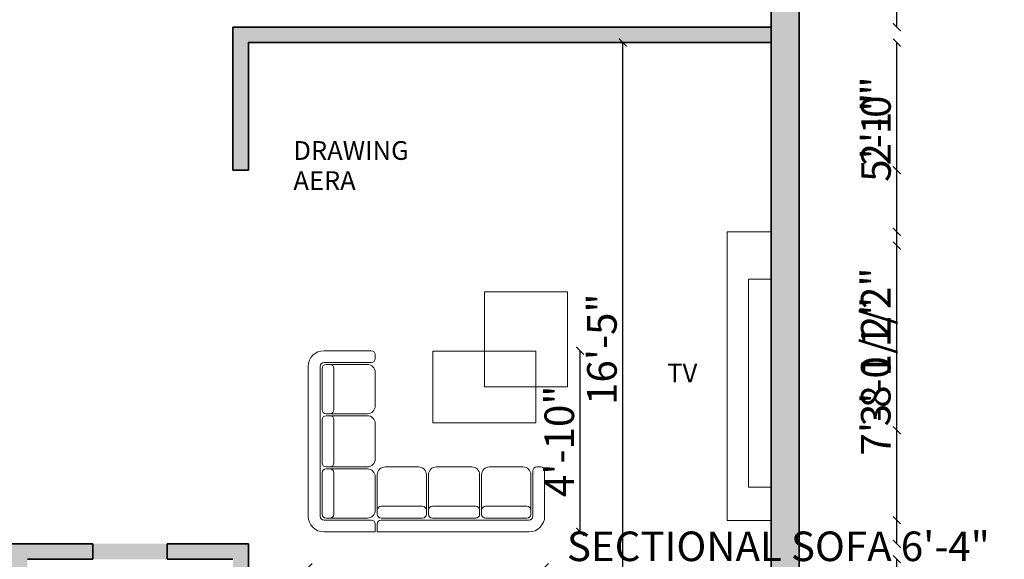
# Model space of a CAD drawing. Units: inches. Extents: x 1704 to 2334, y 1856 to 2559.
# Tile 7 of 10: x 1925 to 2241, y 2148 to 2321. Entities that reach past the tile are written whole.
import ezdxf

# ---------------------------------------------------------------- set-up
doc = ezdxf.new("R2010")
doc.units = ezdxf.units.IN
for name, color, linetype, lineweight in [('A-ANNO-DIMS', 2, 'Continuous', 18), ('A-ANNO-TEXT', 7, 'Continuous', 18), ('A-AREA-IDEN', 7, 'Continuous', 18), ('A-FURN', 8, 'Continuous', 18), ('A-WALL', 7, 'Continuous', 35)]:
    doc.layers.add(name, color=color, linetype=linetype, lineweight=lineweight)
doc.layers.add('A-WALL-PATT', color=18, linetype='Continuous', lineweight=13, true_color=0x000000)
doc.styles.get("Standard").update_dxf_attribs({"font": 'arial.ttf'})
doc.dimstyles.new('ISO-25', dxfattribs={"dimtxt": 9.5, "dimasz": 2.5, "dimexe": 1.25, "dimexo": 0.625, "dimtad": 1, "dimdec": 0, "dimlunit": 4, "dimtxsty": 'Standard', "dimblk": 'ARCHTICK', "dimcen": 2.5, "dimse1": 1, "dimse2": 1, "dimclrd": 3, "dimadec": 0, "dimazin": 0, "dimtfac": 1, "dimtdec": 0, "dimtmove": 0, "dimatfit": 3, "dimfxl": 1, "dimarcsym": 0})

# ---------------------------------------------------------------- blocks, each defined once
blk = doc.blocks.new('A$C2AFA021D')
for p, q in [((0.8, 2.3), (0.2, 2.3)), ((0.85, 2.2), (0.85, 2.25)), ((0.2, 2.15), (0.8, 2.15)), ((0.225, 2.125), (0.275, 2.125)), ((0.75, 2.125), (0.275, 2.125)), ((0, 2.1), (0, 0.2)), ((0.15, 0.2), (0.15, 2.1)), ((0.175, 1.55), (0.175, 2.075)), ((0.325, 2.075), (0.325, 1.55)), ((0.85, 1.6), (0.85, 2.025)), ((0.275, 1.5), (0.225, 1.5)), ((0.275, 1.5), (0.75, 1.5)), ((0.175, 0.875), (0.175, 1.425)), ((0.225, 1.475), (0.275, 1.475)), ((0.75, 1.475), (0.275, 1.475)), ((0.325, 1.425), (0.325, 0.875)), ((0.85, 0.925), (0.85, 1.375)), ((0.175, 0.225), (0.175, 0.75)), ((0.275, 0.825), (0.225, 0.825)), ((0.225, 0.8), (0.275, 0.8)), ((0.275, 0.825), (0.75, 0.825)), ((0.75, 0.8), (0.275, 0.8)), ((0.325, 0.75), (0.325, 0.225)), ((0.975, 0.825), (1.4, 0.825)), ((1.625, 0.825), (2.075, 0.825)), ((2.3, 0.825), (2.725, 0.825)), ((2.85, 0.2), (2.85, 0.775)), ((2.9, 0.825), (2.95, 0.825)), ((3, 0.775), (3, 0.2)), ((0.85, 0.275), (0.85, 0.7)), ((0.875, 0.275), (0.875, 0.725)), ((1.5, 0.725), (1.5, 0.275)), ((1.525, 0.275), (1.525, 0.725)), ((2.175, 0.725), (2.175, 0.275)), ((2.2, 0.275), (2.2, 0.725)), ((2.825, 0.725), (2.825, 0.275)), ((0.875, 0.275), (0.875, 0.225)), ((1.45, 0.325), (0.925, 0.325)), ((1.5, 0.225), (1.5, 0.275)), ((1.525, 0.275), (1.525, 0.225)), ((2.125, 0.325), (1.575, 0.325)), ((2.175, 0.225), (2.175, 0.275)), ((2.2, 0.275), (2.2, 0.225)), ((2.775, 0.325), (2.25, 0.325)), ((2.825, 0.225), (2.825, 0.275)), ((0.8, 0.15), (0.2, 0.15)), ((0.275, 0.175), (0.225, 0.175)), ((0.275, 0.175), (0.75, 0.175)), ((0.925, 0.175), (1.45, 0.175)), ((0.925, 0.15), (2.8, 0.15)), ((1.575, 0.175), (2.125, 0.175)), ((2.25, 0.175), (2.775, 0.175)), ((0.85, 0), (0.85, 0.1)), ((0.875, 0.1), (0.875, 0)), ((0.2, 0), (0.85, 0)), ((2.8, 0), (0.875, 0))]:
    blk.add_line(p, q)
for centre, radius, start, end in [((0.2, 2.1), 0.2, 90, 180), ((0.8, 2.25), 0.05, 0, 90), ((0.2, 2.1), 0.05, 90, 180), ((0.225, 2.075), 0.05, 90, 180), ((0.275, 2.075), 0.05, 0, 90), ((0.75, 2.025), 0.1, 0, 90), ((0.8, 2.2), 0.05, 270, 0), ((0.225, 1.55), 0.05, 180, 270), ((0.275, 1.55), 0.05, 270, 0), ((0.75, 1.6), 0.1, 270, 0), ((0.225, 1.425), 0.05, 90, 180), ((0.275, 1.425), 0.05, 0, 90), ((0.75, 1.375), 0.1, 360, 90), ((0.225, 0.875), 0.05, 180, 270), ((0.275, 0.875), 0.05, 270, 0), ((0.75, 0.925), 0.1, 270, 0), ((0.225, 0.75), 0.05, 90, 180), ((0.275, 0.75), 0.05, 0, 90), ((0.75, 0.7), 0.1, 0, 90), ((0.975, 0.725), 0.1, 90, 180), ((1.4, 0.725), 0.1, 0, 90), ((1.625, 0.725), 0.1, 90, 180), ((2.075, 0.725), 0.1, 0, 90), ((2.3, 0.725), 0.1, 90, 180), ((2.725, 0.725), 0.1, 0, 90), ((2.9, 0.775), 0.05, 90, 180), ((2.95, 0.775), 0.05, 0, 90), ((0.75, 0.275), 0.1, 270, 0), ((0.925, 0.275), 0.05, 90, 180), ((1.45, 0.275), 0.05, 360, 90), ((1.575, 0.275), 0.05, 90, 180), ((2.125, 0.275), 0.05, 360, 90), ((2.25, 0.275), 0.05, 90, 180), ((2.775, 0.275), 0.05, 360, 90), ((0.2, 0.2), 0.2, 180, 270), ((0.2, 0.2), 0.05, 180, 270), ((0.225, 0.225), 0.05, 180, 270), ((0.275, 0.225), 0.05, 270, 0), ((0.8, 0.1), 0.05, 0, 90), ((0.925, 0.225), 0.05, 180, 270), ((0.925, 0.1), 0.05, 90, 180), ((1.45, 0.225), 0.05, 270, 0), ((1.575, 0.225), 0.05, 180, 270), ((2.125, 0.225), 0.05, 270, 0), ((2.25, 0.225), 0.05, 180, 270), ((2.775, 0.225), 0.05, 270, 0), ((2.8, 0.2), 0.2, 270, 0), ((2.8, 0.2), 0.05, 270, 0)]:
    blk.add_arc(centre, radius, start, end)
blk = doc.blocks.new('_ArchTick')
at = {"color": 0, "linetype": 'ByBlock', "const_width": 0.15}
blk.add_lwpolyline([(-0.5, -0.5), (0.5, 0.5)], dxfattribs=at)
blk = doc.blocks.new('*D21')
at = {"layer": 'A-ANNO-DIMS', "color": 0, "lineweight": -2, "transparency": 16777216}
blk.add_line((2118.31, 2117.04), (2118.31, 2314.04), dxfattribs=at)
at = {"layer": 'Defpoints', "color": 0, "transparency": 16777216}
for p in [(2118.31, 2314.04), (2129.02, 2314.04), (2129.02, 2117.04)]:
    blk.add_point(p, dxfattribs=at)
at = {"layer": 'A-ANNO-DIMS', "color": 0, "lineweight": -2, "transparency": 16777216, "xscale": 2.5, "yscale": 2.5, "zscale": 2.5}
for p, rotation in [((2118.31, 2314.04), 90), ((2118.31, 2117.04), 270)]:
    blk.add_blockref('_ArchTick', p, dxfattribs=dict(at, rotation=rotation))
at = {"layer": 'A-ANNO-DIMS', "color": 0, "transparency": 16777216, "insert": (2112.83, 2215.54), "char_height": 9.5, "attachment_point": 5, "rotation": 90}
blk.add_mtext('16\'-5"', dxfattribs=at)
blk = doc.blocks.new('*D26')
at = {"layer": 'A-ANNO-DIMS', "color": 3, "lineweight": -2, "transparency": 16777216}
for p, q in [((2017.24, 2145.44), (2093.2, 2145.44)), ((2093.2, 2145.44), (2240.89, 2145.44))]:
    blk.add_line(p, q, dxfattribs=at)
at = {"layer": 'Defpoints', "color": 0, "transparency": 16777216}
for p in [(2017.24, 2156.83), (2093.2, 2156.83), (2093.2, 2145.44)]:
    blk.add_point(p, dxfattribs=at)
at = {"layer": 'A-ANNO-DIMS', "color": 3, "lineweight": -2, "transparency": 16777216, "xscale": 2.5, "yscale": 2.5, "zscale": 2.5, "rotation": 180}
blk.add_blockref('_ArchTick', (2017.24, 2145.44), dxfattribs=at)
at = {"layer": 'A-ANNO-DIMS', "color": 3, "lineweight": -2, "transparency": 16777216, "xscale": 2.5, "yscale": 2.5, "zscale": 2.5}
blk.add_blockref('_ArchTick', (2093.2, 2145.44), dxfattribs=at)
at = {"layer": 'A-ANNO-DIMS', "color": 0, "transparency": 16777216, "insert": (2168.29, 2150.98), "char_height": 9.5, "attachment_point": 5}
blk.add_mtext('SECTIONAL SOFA 6\'-4"', dxfattribs=at)
blk = doc.blocks.new('*D27')
at = {"layer": 'A-ANNO-DIMS', "color": 3, "lineweight": -2, "transparency": 16777216}
blk.add_line((2104.59, 2156.83), (2104.59, 2215.06), dxfattribs=at)
at = {"layer": 'Defpoints', "color": 0, "transparency": 16777216}
for p in [(2093.2, 2215.06), (2104.59, 2215.06), (2093.2, 2156.83)]:
    blk.add_point(p, dxfattribs=at)
at = {"layer": 'A-ANNO-DIMS', "color": 3, "lineweight": -2, "transparency": 16777216, "xscale": 2.5, "yscale": 2.5, "zscale": 2.5}
for p, rotation in [((2104.59, 2215.06), 90), ((2104.59, 2156.83), 270)]:
    blk.add_blockref('_ArchTick', p, dxfattribs=dict(at, rotation=rotation))
at = {"layer": 'A-ANNO-DIMS', "color": 0, "transparency": 16777216, "insert": (2099.12, 2185.95), "char_height": 9.5, "attachment_point": 5, "rotation": 90}
blk.add_mtext('4\'-10"', dxfattribs=at)
blk = doc.blocks.new('*D36')
at = {"layer": 'A-ANNO-DIMS', "color": 3, "lineweight": -2, "transparency": 16777216}
blk.add_line((2206.36, 2319.04), (2206.36, 2499.04), dxfattribs=at)
at = {"layer": 'Defpoints', "color": 0, "transparency": 16777216}
for p in [(2166.01, 2499.04), (2206.36, 2499.04), (2166.01, 2319.04)]:
    blk.add_point(p, dxfattribs=at)
at = {"layer": 'A-ANNO-DIMS', "color": 3, "lineweight": -2, "transparency": 16777216, "xscale": 2.5, "yscale": 2.5, "zscale": 2.5}
for p, rotation in [((2206.36, 2499.04), 90), ((2206.36, 2319.04), 270)]:
    blk.add_blockref('_ArchTick', p, dxfattribs=dict(at, rotation=rotation))
at = {"layer": 'A-ANNO-DIMS', "color": 0, "transparency": 16777216, "insert": (2200.88, 2409.04), "char_height": 9.5, "attachment_point": 5, "rotation": 90}
blk.add_mtext('15\'-0"', dxfattribs=at)
blk = doc.blocks.new('*D39')
at = {"layer": 'A-ANNO-DIMS', "color": 3, "lineweight": -2, "transparency": 16777216}
blk.add_line((2206.36, 2074.24), (2206.36, 2148.04), dxfattribs=at)
at = {"layer": 'Defpoints', "color": 0, "transparency": 16777216}
for p in [(1927.01, 2148.04), (2206.36, 2148.04), (1927.01, 2074.24)]:
    blk.add_point(p, dxfattribs=at)
at = {"layer": 'A-ANNO-DIMS', "color": 3, "lineweight": -2, "transparency": 16777216, "xscale": 2.5, "yscale": 2.5, "zscale": 2.5}
for p, rotation in [((2206.36, 2148.04), 90), ((2206.36, 2074.24), 270)]:
    blk.add_blockref('_ArchTick', p, dxfattribs=dict(at, rotation=rotation))
at = {"layer": 'A-ANNO-DIMS', "color": 0, "transparency": 16777216, "insert": (2200.88, 2111.14), "char_height": 9.5, "attachment_point": 5, "rotation": 90}
blk.add_mtext('6\'-2"', dxfattribs=at)
blk = doc.blocks.new('*D46')
at = {"layer": 'A-ANNO-DIMS', "color": 3, "lineweight": -2, "transparency": 16777216}
for p, q in [((2206.36, 2189.49), (2206.36, 2240.62)), ((2206.36, 2153.04), (2206.36, 2189.49))]:
    blk.add_line(p, q, dxfattribs=at)
at = {"layer": 'Defpoints', "color": 0, "transparency": 16777216}
for p in [(1886.55, 2189.49), (2206.36, 2189.49), (1886.55, 2153.04)]:
    blk.add_point(p, dxfattribs=at)
at = {"layer": 'A-ANNO-DIMS', "color": 3, "lineweight": -2, "transparency": 16777216, "xscale": 2.5, "yscale": 2.5, "zscale": 2.5}
for p, rotation in [((2206.36, 2189.49), 90), ((2206.36, 2153.04), 270)]:
    blk.add_blockref('_ArchTick', p, dxfattribs=dict(at, rotation=rotation))
at = {"layer": 'A-ANNO-DIMS', "color": 0, "transparency": 16777216, "insert": (2200.82, 2216.3), "char_height": 9.5, "attachment_point": 5, "rotation": 90}
blk.add_mtext('3\'-0 1/2"', dxfattribs=at)
blk = doc.blocks.new('*D47')
at = {"layer": 'A-ANNO-DIMS', "color": 3, "lineweight": -2, "transparency": 16777216}
for p, q in [((2206.36, 2273.04), (2206.36, 2302.2)), ((2206.36, 2248.82), (2206.36, 2273.04))]:
    blk.add_line(p, q, dxfattribs=at)
at = {"layer": 'Defpoints', "color": 0, "transparency": 16777216}
for p in [(1900.32, 2273.04), (2206.36, 2273.04), (1900.32, 2248.82)]:
    blk.add_point(p, dxfattribs=at)
at = {"layer": 'A-ANNO-DIMS', "color": 3, "lineweight": -2, "transparency": 16777216, "xscale": 2.5, "yscale": 2.5, "zscale": 2.5}
for p, rotation in [((2206.36, 2273.04), 90), ((2206.36, 2248.82), 270)]:
    blk.add_blockref('_ArchTick', p, dxfattribs=dict(at, rotation=rotation))
at = {"layer": 'A-ANNO-DIMS', "color": 0, "transparency": 16777216, "insert": (2200.88, 2288.87), "char_height": 9.5, "attachment_point": 5, "rotation": 90}
blk.add_mtext('2\'-0"', dxfattribs=at)
blk = doc.blocks.new('*D49')
at = {"layer": 'A-ANNO-DIMS', "color": 3, "lineweight": -2, "transparency": 16777216}
for p, q in [((1998.01, 2539.39), (2017.2, 2539.39)), ((2017.2, 2539.39), (2045.31, 2539.39))]:
    blk.add_line(p, q, dxfattribs=at)
at = {"layer": 'Defpoints', "color": 0, "transparency": 16777216}
for p in [(2017.2, 2539.39), (1998.01, 2117.04), (2017.2, 2117.04)]:
    blk.add_point(p, dxfattribs=at)
at = {"layer": 'A-ANNO-DIMS', "color": 3, "lineweight": -2, "transparency": 16777216, "xscale": 2.5, "yscale": 2.5, "zscale": 2.5, "rotation": 180}
blk.add_blockref('_ArchTick', (1998.01, 2539.39), dxfattribs=at)
at = {"layer": 'A-ANNO-DIMS', "color": 3, "lineweight": -2, "transparency": 16777216, "xscale": 2.5, "yscale": 2.5, "zscale": 2.5}
blk.add_blockref('_ArchTick', (2017.2, 2539.39), dxfattribs=at)
at = {"layer": 'A-ANNO-DIMS', "color": 0, "transparency": 16777216, "insert": (2032.51, 2544.78), "char_height": 9.5, "attachment_point": 5}
blk.add_mtext('1\'-7"', dxfattribs=at)
blk = doc.blocks.new('*D50')
at = {"layer": 'A-ANNO-DIMS', "color": 3, "lineweight": -2, "transparency": 16777216}
blk.add_line((2017.2, 2539.39), (2045.28, 2539.39), dxfattribs=at)
at = {"layer": 'Defpoints', "color": 0, "transparency": 16777216}
for p in [(2045.28, 2539.39), (2017.2, 2117.04), (2045.28, 2117.04)]:
    blk.add_point(p, dxfattribs=at)
at = {"layer": 'A-ANNO-DIMS', "color": 3, "lineweight": -2, "transparency": 16777216, "xscale": 2.5, "yscale": 2.5, "zscale": 2.5, "rotation": 180}
blk.add_blockref('_ArchTick', (2017.2, 2539.39), dxfattribs=at)
at = {"layer": 'A-ANNO-DIMS', "color": 3, "lineweight": -2, "transparency": 16777216, "xscale": 2.5, "yscale": 2.5, "zscale": 2.5}
blk.add_blockref('_ArchTick', (2045.28, 2539.39), dxfattribs=at)
at = {"layer": 'A-ANNO-DIMS', "color": 0, "transparency": 16777216, "insert": (2031.24, 2544.78), "char_height": 9.5, "attachment_point": 5}
blk.add_mtext('2\'-4"', dxfattribs=at)
blk = doc.blocks.new('*D51')
at = {"layer": 'A-ANNO-DIMS', "color": 3, "lineweight": -2, "transparency": 16777216}
for p, q in [((2045.28, 2539.39), (2054.53, 2539.39)), ((2054.53, 2539.39), (2105.67, 2539.39))]:
    blk.add_line(p, q, dxfattribs=at)
at = {"layer": 'Defpoints', "color": 0, "transparency": 16777216}
for p in [(2054.53, 2539.39), (2045.28, 2117.04), (2054.53, 2117.04)]:
    blk.add_point(p, dxfattribs=at)
at = {"layer": 'A-ANNO-DIMS', "color": 3, "lineweight": -2, "transparency": 16777216, "xscale": 2.5, "yscale": 2.5, "zscale": 2.5, "rotation": 180}
blk.add_blockref('_ArchTick', (2045.28, 2539.39), dxfattribs=at)
at = {"layer": 'A-ANNO-DIMS', "color": 3, "lineweight": -2, "transparency": 16777216, "xscale": 2.5, "yscale": 2.5, "zscale": 2.5}
blk.add_blockref('_ArchTick', (2054.53, 2539.39), dxfattribs=at)
at = {"layer": 'A-ANNO-DIMS', "color": 0, "transparency": 16777216, "insert": (2081.35, 2544.93), "char_height": 9.5, "attachment_point": 5}
blk.add_mtext('0\'-9 1/2"', dxfattribs=at)
blk = doc.blocks.new('*D52')
at = {"layer": 'A-ANNO-DIMS', "color": 3, "lineweight": -2, "transparency": 16777216}
blk.add_line((2054.53, 2539.39), (2105.53, 2539.39), dxfattribs=at)
at = {"layer": 'Defpoints', "color": 0, "transparency": 16777216}
for p in [(2105.53, 2539.39), (2054.53, 2117.04), (2105.53, 2117.04)]:
    blk.add_point(p, dxfattribs=at)
at = {"layer": 'A-ANNO-DIMS', "color": 3, "lineweight": -2, "transparency": 16777216, "xscale": 2.5, "yscale": 2.5, "zscale": 2.5, "rotation": 180}
blk.add_blockref('_ArchTick', (2054.53, 2539.39), dxfattribs=at)
at = {"layer": 'A-ANNO-DIMS', "color": 3, "lineweight": -2, "transparency": 16777216, "xscale": 2.5, "yscale": 2.5, "zscale": 2.5}
blk.add_blockref('_ArchTick', (2105.53, 2539.39), dxfattribs=at)
at = {"layer": 'A-ANNO-DIMS', "color": 0, "transparency": 16777216, "insert": (2080.03, 2544.87), "char_height": 9.5, "attachment_point": 5}
blk.add_mtext('4\'-3"', dxfattribs=at)
blk = doc.blocks.new('*D64')
at = {"layer": 'A-ANNO-DIMS', "color": 3, "lineweight": -2, "transparency": 16777216}
for p, q in [((1948.02, 2539.39), (1971.87, 2539.39)), ((1971.87, 2539.39), (2001.04, 2539.39))]:
    blk.add_line(p, q, dxfattribs=at)
at = {"layer": 'Defpoints', "color": 0, "transparency": 16777216}
for p in [(1971.87, 2539.39), (1948.02, 2153.04), (1971.87, 2153.04)]:
    blk.add_point(p, dxfattribs=at)
at = {"layer": 'A-ANNO-DIMS', "color": 3, "lineweight": -2, "transparency": 16777216, "xscale": 2.5, "yscale": 2.5, "zscale": 2.5, "rotation": 180}
blk.add_blockref('_ArchTick', (1948.02, 2539.39), dxfattribs=at)
at = {"layer": 'A-ANNO-DIMS', "color": 3, "lineweight": -2, "transparency": 16777216, "xscale": 2.5, "yscale": 2.5, "zscale": 2.5}
blk.add_blockref('_ArchTick', (1971.87, 2539.39), dxfattribs=at)
at = {"layer": 'A-ANNO-DIMS', "color": 0, "transparency": 16777216, "insert": (1987.71, 2544.86), "char_height": 9.5, "attachment_point": 5}
blk.add_mtext('2\'-0"', dxfattribs=at)
blk = doc.blocks.new('*D74')
at = {"layer": 'A-ANNO-DIMS', "color": 3, "lineweight": -2, "transparency": 16777216}
blk.add_line((1916.93, 2539.39), (1948.02, 2539.39), dxfattribs=at)
at = {"layer": 'Defpoints', "color": 0, "transparency": 16777216}
for p in [(1948.02, 2539.39), (1916.93, 2153.04), (1948.02, 2153.04)]:
    blk.add_point(p, dxfattribs=at)
at = {"layer": 'A-ANNO-DIMS', "color": 3, "lineweight": -2, "transparency": 16777216, "xscale": 2.5, "yscale": 2.5, "zscale": 2.5, "rotation": 180}
blk.add_blockref('_ArchTick', (1916.93, 2539.39), dxfattribs=at)
at = {"layer": 'A-ANNO-DIMS', "color": 3, "lineweight": -2, "transparency": 16777216, "xscale": 2.5, "yscale": 2.5, "zscale": 2.5}
blk.add_blockref('_ArchTick', (1948.02, 2539.39), dxfattribs=at)
at = {"layer": 'A-ANNO-DIMS', "color": 0, "transparency": 16777216, "insert": (1932.47, 2544.78), "char_height": 9.5, "attachment_point": 5}
blk.add_mtext('2\'-7"', dxfattribs=at)
blk = doc.blocks.new('*D78')
at = {"layer": 'A-ANNO-DIMS', "color": 3, "lineweight": -2, "transparency": 16777216}
blk.add_line((1723.66, 2273.04), (1723.66, 2319.04), dxfattribs=at)
at = {"layer": 'Defpoints', "color": 0, "transparency": 16777216}
for p in [(1723.66, 2319.04), (1993.01, 2319.04), (1993.01, 2273.04)]:
    blk.add_point(p, dxfattribs=at)
at = {"layer": 'A-ANNO-DIMS', "color": 3, "lineweight": -2, "transparency": 16777216, "xscale": 2.5, "yscale": 2.5, "zscale": 2.5}
for p, rotation in [((1723.66, 2319.04), 90), ((1723.66, 2273.04), 270)]:
    blk.add_blockref('_ArchTick', p, dxfattribs=dict(at, rotation=rotation))
at = {"layer": 'A-ANNO-DIMS', "color": 0, "transparency": 16777216, "insert": (1718.18, 2296.04), "char_height": 9.5, "attachment_point": 5, "rotation": 90}
blk.add_mtext('3\'-10"', dxfattribs=at)
blk = doc.blocks.new('*D79')
at = {"layer": 'A-ANNO-DIMS', "color": 3, "lineweight": -2, "transparency": 16777216}
blk.add_line((1723.66, 2350.04), (1723.66, 2319.04), dxfattribs=at)
at = {"layer": 'Defpoints', "color": 0, "transparency": 16777216}
for p in [(1998.01, 2350.04), (1723.66, 2319.04), (1993.01, 2319.04)]:
    blk.add_point(p, dxfattribs=at)
at = {"layer": 'A-ANNO-DIMS', "color": 3, "lineweight": -2, "transparency": 16777216, "xscale": 2.5, "yscale": 2.5, "zscale": 2.5}
for p, rotation in [((1723.66, 2350.04), 90), ((1723.66, 2319.04), 270)]:
    blk.add_blockref('_ArchTick', p, dxfattribs=dict(at, rotation=rotation))
at = {"layer": 'A-ANNO-DIMS', "color": 0, "transparency": 16777216, "insert": (1718.27, 2334.54), "char_height": 9.5, "attachment_point": 5, "rotation": 90}
blk.add_mtext('2\'-7"', dxfattribs=at)
blk = doc.blocks.new('*D80')
at = {"layer": 'A-ANNO-DIMS', "color": 3, "lineweight": -2, "transparency": 16777216}
blk.add_line((1900.32, 2539.39), (1993.01, 2539.39), dxfattribs=at)
at = {"layer": 'Defpoints', "color": 0, "transparency": 16777216}
for p in [(1993.01, 2539.39), (1900.32, 2273.04), (1993.01, 2273.04)]:
    blk.add_point(p, dxfattribs=at)
at = {"layer": 'A-ANNO-DIMS', "color": 3, "lineweight": -2, "transparency": 16777216, "xscale": 2.5, "yscale": 2.5, "zscale": 2.5, "rotation": 180}
blk.add_blockref('_ArchTick', (1900.32, 2539.39), dxfattribs=at)
at = {"layer": 'A-ANNO-DIMS', "color": 3, "lineweight": -2, "transparency": 16777216, "xscale": 2.5, "yscale": 2.5, "zscale": 2.5}
blk.add_blockref('_ArchTick', (1993.01, 2539.39), dxfattribs=at)
at = {"layer": 'A-ANNO-DIMS', "color": 0, "transparency": 16777216, "insert": (1946.66, 2544.93), "char_height": 9.5, "attachment_point": 5}
blk.add_mtext('7\'-8 1/2"', dxfattribs=at)
blk = doc.blocks.new('*D81')
at = {"layer": 'A-ANNO-DIMS', "color": 3, "lineweight": -2, "transparency": 16777216}
blk.add_line((2206.36, 2074.93), (2206.36, 2148.04), dxfattribs=at)
at = {"layer": 'Defpoints', "color": 0, "transparency": 16777216}
for p in [(1796.13, 2148.04), (2206.36, 2148.04), (1790.01, 2074.93)]:
    blk.add_point(p, dxfattribs=at)
at = {"layer": 'A-ANNO-DIMS', "color": 3, "lineweight": -2, "transparency": 16777216, "xscale": 2.5, "yscale": 2.5, "zscale": 2.5}
for p, rotation in [((2206.36, 2148.04), 90), ((2206.36, 2074.93), 270)]:
    blk.add_blockref('_ArchTick', p, dxfattribs=dict(at, rotation=rotation))
at = {"layer": 'A-ANNO-DIMS', "color": 0, "transparency": 16777216, "insert": (2200.88, 2111.48), "char_height": 9.5, "attachment_point": 5, "rotation": 90}
blk.add_mtext('6\'-1"', dxfattribs=at)
blk = doc.blocks.new('*D86')
at = {"layer": 'A-ANNO-DIMS', "color": 3, "lineweight": -2, "transparency": 16777216}
blk.add_line((2206.36, 2160.56), (2206.36, 2253.22), dxfattribs=at)
at = {"layer": 'Defpoints', "color": 0, "transparency": 16777216}
for p in [(2166.01, 2253.22), (2206.36, 2253.22), (2166.01, 2160.56)]:
    blk.add_point(p, dxfattribs=at)
at = {"layer": 'A-ANNO-DIMS', "color": 3, "lineweight": -2, "transparency": 16777216, "xscale": 2.5, "yscale": 2.5, "zscale": 2.5}
for p, rotation in [((2206.36, 2253.22), 90), ((2206.36, 2160.56), 270)]:
    blk.add_blockref('_ArchTick', p, dxfattribs=dict(at, rotation=rotation))
at = {"layer": 'A-ANNO-DIMS', "color": 0, "transparency": 16777216, "insert": (2200.82, 2206.89), "char_height": 9.5, "attachment_point": 5, "rotation": 90}
blk.add_mtext('7\'-8 1/2"', dxfattribs=at)
blk = doc.blocks.new('*D87')
at = {"layer": 'A-ANNO-DIMS', "color": 3, "lineweight": -2, "transparency": 16777216}
blk.add_line((2206.36, 2253.22), (2206.36, 2314.04), dxfattribs=at)
at = {"layer": 'Defpoints', "color": 0, "transparency": 16777216}
for p in [(2166.01, 2314.04), (2206.36, 2314.04), (2166.01, 2253.22)]:
    blk.add_point(p, dxfattribs=at)
at = {"layer": 'A-ANNO-DIMS', "color": 3, "lineweight": -2, "transparency": 16777216, "xscale": 2.5, "yscale": 2.5, "zscale": 2.5}
for p, rotation in [((2206.36, 2314.04), 90), ((2206.36, 2253.22), 270)]:
    blk.add_blockref('_ArchTick', p, dxfattribs=dict(at, rotation=rotation))
at = {"layer": 'A-ANNO-DIMS', "color": 0, "transparency": 16777216, "insert": (2200.88, 2283.63), "char_height": 9.5, "attachment_point": 5, "rotation": 90}
blk.add_mtext('5\'-1"', dxfattribs=at)

msp = doc.modelspace()

# ---------------------------------------------------------------- hatches: boundary and pattern name
at = {"layer": 'A-WALL-PATT'}
h = msp.add_hatch(color=256, dxfattribs=at)
h.dxf.hatch_style = 1
h.paths.add_polyline_path([(1764.01, 2204.96), (1755.01, 2204.96), (1755.01, 2115.31), (1764.01, 2115.31)])
h.paths.add_polyline_path([(1764.01, 2076.84), (1755.01, 2076.84), (1755.01, 1968.04), (1794.77, 1968.04), (1794.77, 1977.04), (1764.01, 1977.04)])
h.paths.add_polyline_path([(1927.01, 1977.04), (1927.01, 2069.24), (1993.01, 2069.24), (1993.01, 1977.04)], flags=16)
h.paths.add_polyline_path([(1927.01, 2074.24), (1927.01, 2148.04), (1993.01, 2148.04), (1993.01, 2074.24)], flags=16)
h.paths.add_polyline_path([(1764.01, 2318.65), (1755.01, 2318.65), (1755.01, 2247.44), (1764.01, 2247.44)])
h.paths.add_polyline_path([(1764.01, 2499.04), (1798.75, 2499.04), (1798.75, 2508.04), (1755.01, 2508.04), (1755.01, 2336.43), (1764.01, 2336.43)])
h.paths.add_polyline_path([(1950.56, 2508.04), (1847.17, 2508.04), (1847.17, 2499.04), (1950.56, 2499.04)])
h.paths.add_polyline_path([(2059.64, 2508.04), (1975.68, 2508.04), (1975.68, 2499.04), (2059.64, 2499.04)])
h.paths.add_polyline_path([(2175.01, 2508.04), (2108.25, 2508.04), (2108.25, 2499.04), (2166.01, 2499.04), (2166.01, 1977.04), (2166.01, 1972.26), (2166.01, 1968.04), (2175.01, 1968.04)])
h.paths.add_polyline_path([(2166.01, 2319.04), (1993.01, 2319.04), (1993.01, 2273.04), (1998.01, 2273.04), (1998.01, 2314.04), (2166.01, 2314.04)])
h.paths.add_polyline_path([(2054.53, 2117.04), (1998.01, 2117.04), (1998.01, 2112.04), (2054.53, 2112.04)])
h.paths.add_polyline_path([(2166.01, 2117.04), (2105.53, 2117.04), (2105.53, 2112.04), (2166.01, 2112.04)])
h.paths.add_polyline_path([(1927.01, 2499.04), (1922.01, 2499.04), (1922.01, 2355.04), (1764.01, 2355.04), (1764.01, 2350.04), (1804.01, 2350.04), (1804.01, 2278.04), (1764.01, 2278.04), (1764.01, 2273.04), (1870.51, 2273.04), (1870.51, 2278.04), (1870.51, 2350.04), (1865.51, 2350.04), (1865.51, 2278.04), (1809.01, 2278.04), (1809.01, 2350.04), (1922.01, 2350.04), (1927.01, 2350.04), (1998.01, 2350.04), (1998.01, 2499.04), (1993.01, 2499.04), (1993.01, 2355.04), (1927.01, 2355.04)])
h.paths.add_polyline_path([(2131.1, 2203.36), (2144.85, 2203.36), (2144.85, 2212.38), (2131.1, 2212.38)], flags=25)
h.paths.add_polyline_path([(2010.94, 2265.21), (2036.85, 2265.21), (2036.85, 2274.23), (2010.94, 2274.23)], flags=9)
h.paths.add_polyline_path([(2010.9, 2274.71), (2056.95, 2274.71), (2056.95, 2284.04), (2010.9, 2284.04)], flags=25)
h.paths.add_polyline_path([(2003.27, 2440.18), (2049.79, 2440.18), (2049.79, 2449.51), (2003.27, 2449.51)], flags=9)
h.paths.add_polyline_path([(1934.96, 2428.22), (1967.48, 2428.22), (1967.48, 2437.55), (1934.96, 2437.55)], flags=25)
h.paths.add_polyline_path([(1778.93, 2466.23), (1827.79, 2466.23), (1827.79, 2475.56), (1778.93, 2475.56)], flags=25)
h.paths.add_polyline_path([(1938.32, 2043.05), (1970.37, 2043.05), (1970.37, 2052.39), (1938.32, 2052.39)], flags=8)
h.paths.add_polyline_path([(1932.21, 2095.38), (1956.75, 2095.38), (1956.75, 2104.56), (1932.21, 2104.56)], flags=8)
h.paths.add_polyline_path([(1888.97, 2148.04), (1888.97, 2153.04), (1764.01, 2153.04), (1764.01, 2148.04)])
h.paths.add_polyline_path([(1922.01, 2059.61), (1927.01, 2059.61), (1927.01, 2044.47), (1922.01, 2044.47), (1922.01, 1977.04), (1857.04, 1977.04), (1857.04, 1968.04), (1998.01, 1968.04), (1998.01, 1977.04), (1998.01, 2153.04), (1916.93, 2153.04), (1916.93, 2148.04), (1922.01, 2148.04)])

# ---------------------------------------------------------------- linework, layer by layer
at = {"layer": 'A-FURN'}
for points in [[(2166.01, 2253.22), (2151.89, 2253.22), (2151.89, 2160.56), (2166.01, 2160.56)], [(2166.01, 2238.04), (2158.69, 2238.04), (2158.69, 2171.17), (2166.01, 2171.17)], [(2073.86, 2203.43), (2100.5, 2203.43), (2100.5, 2233.99), (2073.86, 2233.99)], [(2057.31, 2214.95), (2090.4, 2214.95), (2090.4, 2191.92), (2057.31, 2191.92)]]:
    msp.add_lwpolyline(points, close=True, dxfattribs=at)
at = {"layer": 'A-WALL'}
for p, q in [((2166.01, 2499.04), (2166.01, 1977.04)), ((1993.01, 2319.04), (2166.01, 2319.04)), ((1993.01, 2273.04), (1993.01, 2319.04)), ((1993.01, 2319.04), (1993.01, 2314.04)), ((1998.01, 2314.04), (2166.01, 2314.04)), ((1998.01, 2273.04), (1998.01, 2314.04)), ((1993.01, 2273.04), (1998.01, 2273.04)), ((1764.01, 2153.04), (1948.02, 2153.04)), ((1948.02, 2153.04), (1948.02, 2148.04)), ((1948.02, 2153.04), (1948.02, 2148.04)), ((1971.87, 2153.04), (1971.87, 2148.04)), ((1971.87, 2153.04), (1998.01, 2153.04)), ((1998.01, 1977.04), (1998.01, 2153.04)), ((1927.01, 2148.04), (1948.02, 2148.04)), ((1971.87, 2148.04), (1993.01, 2148.04))]:
    msp.add_line(p, q, dxfattribs=at)
msp.add_lwpolyline([(1998.01, 1968.04), (1755.01, 1968.04), (1755.01, 2508.04), (2175.01, 2508.04), (2175.01, 1968.04), (2166.01, 1968.04)], dxfattribs=at)

# ---------------------------------------------------------------- block references
at = {"layer": 'A-FURN', "xscale": 25.31830499288571, "yscale": 25.31830499288571, "zscale": 25.31830499288571}
msp.add_blockref('A$C2AFA021D', (2017.24, 2156.83), dxfattribs=at)

# ---------------------------------------------------------------- texts
at = {"layer": 'A-ANNO-TEXT'}
msp.add_text('TV', height=6.013, dxfattribs=at).set_placement((2132.61, 2204.86))
at = {"layer": 'A-AREA-IDEN'}
for s, p in [('DRAWING ', (2012.46, 2276.37)), ('AERA', (2012.46, 2266.71))]:
    msp.add_text(s, height=6.013, dxfattribs=at).set_placement(p)

# ---------------------------------------------------------------- dimensions: what is measured, and where the dimension line sits
at = {"layer": 'A-ANNO-DIMS'}
for base, p1, p2, picture, middle in [((1993.01, 2539.39), (1900.32, 2273.04), (1993.01, 2273.04), '*D80', (1946.66, 2544.93)), ((2054.5307, 2539.3895), (2045.2758, 2117.0395), (2054.5307, 2117.0395), '*D51', (2081.3506, 2544.9265)), ((1948.02, 2539.39), (1916.93, 2153.04), (1948.02, 2153.04), '*D74', (1932.47, 2544.78)), ((1971.8732, 2539.3895), (1948.0187, 2153.0395), (1971.8732, 2153.0395), '*D64', (1987.7059, 2544.8649)), ((2017.2, 2539.39), (1998.01, 2117.04), (2017.2, 2117.04), '*D49', (2032.51, 2544.78)), ((2045.28, 2539.39), (2017.2, 2117.04), (2045.28, 2117.04), '*D50', (2031.24, 2544.78)), ((2105.53, 2539.39), (2054.53, 2117.04), (2105.53, 2117.04), '*D52', (2080.03, 2544.87))]:
    dim = msp.add_linear_dim(base=base, p1=p1, p2=p2, dimstyle='ISO-25', override={"dimdec": 1, "dimlfac": 1, "dimrnd": 0, "dimzin": 1, "dimdsep": 46, "dimlunit": 4, "dimfrac": 2}, dxfattribs=at)
    dim.commit()
    dim.dimension.update_dxf_attribs({"geometry": picture, "text_midpoint": middle})
for base, p1, p2, override, picture, middle in [((2206.36, 2499.04), (2166.01, 2319.04), (2166.01, 2499.04), {"dimdec": 1, "dimlfac": 1, "dimrnd": 0, "dimzin": 1, "dimdsep": 46, "dimlunit": 4, "dimfrac": 2}, '*D36', (2200.88, 2409.04)), ((1723.66, 2319.04), (1998.01, 2350.04), (1993.01, 2319.04), {"dimdec": 1, "dimlfac": 1, "dimrnd": 0, "dimzin": 1, "dimdsep": 46, "dimlunit": 4, "dimfrac": 2}, '*D79', (1718.27, 2334.54)), ((1723.66, 2319.04), (1993.01, 2273.04), (1993.01, 2319.04), {"dimdec": 1, "dimlfac": 1, "dimrnd": 0, "dimzin": 1, "dimdsep": 46, "dimlunit": 4, "dimfrac": 2}, '*D78', (1718.18, 2296.04)), ((2118.31, 2314.04), (2129.02, 2117.04), (2129.02, 2314.04), {"dimclrd": 0, "dimclre": 0, "dimclrt": 0}, '*D21', (2112.83, 2215.54)), ((2206.36, 2314.04), (2166.01, 2253.22), (2166.01, 2314.04), {"dimdec": 1, "dimlfac": 1, "dimrnd": 0, "dimzin": 1, "dimdsep": 46, "dimlunit": 4, "dimfrac": 2}, '*D87', (2200.88, 2283.63)), ((2206.36, 2273.04), (1900.32, 2248.82), (1900.32, 2273.04), {"dimdec": 1, "dimlfac": 1, "dimrnd": 0, "dimzin": 1, "dimdsep": 46, "dimlunit": 4, "dimfrac": 2}, '*D47', (2200.88, 2288.87)), ((2206.36, 2253.22), (2166.01, 2160.56), (2166.01, 2253.22), {"dimdec": 1, "dimlfac": 1, "dimrnd": 0, "dimzin": 1, "dimdsep": 46, "dimlunit": 4, "dimfrac": 2}, '*D86', (2200.82, 2206.89)), ((2206.3597, 2189.4875), (1886.552, 2153.0395), (1886.552, 2189.4875), {"dimdec": 1, "dimlfac": 1, "dimrnd": 0, "dimzin": 1, "dimdsep": 46, "dimlunit": 4, "dimfrac": 2}, '*D46', (2200.8195, 2216.3042)), ((2104.59, 2215.06), (2093.2, 2156.83), (2093.2, 2215.06), {"dimdec": 1, "dimlfac": 1, "dimrnd": 0, "dimzin": 1, "dimdsep": 46, "dimlunit": 4, "dimfrac": 2}, '*D27', (2099.12, 2185.95)), ((2206.36, 2148.04), (1790.01, 2074.93), (1796.13, 2148.04), {"dimdec": 1, "dimlfac": 1, "dimrnd": 0, "dimzin": 1, "dimdsep": 46, "dimlunit": 4, "dimfrac": 2}, '*D81', (2200.88, 2111.48)), ((2206.36, 2148.04), (1927.01, 2074.24), (1927.01, 2148.04), {"dimdec": 1, "dimlfac": 1, "dimrnd": 0, "dimzin": 1, "dimdsep": 46, "dimlunit": 4, "dimfrac": 2}, '*D39', (2200.88, 2111.14))]:
    dim = msp.add_linear_dim(base=base, p1=p1, p2=p2, angle=90, dimstyle='ISO-25', override=override, dxfattribs=at)
    dim.commit()
    dim.dimension.update_dxf_attribs({"geometry": picture, "text_midpoint": middle})
dim = msp.add_linear_dim(base=(2093.2, 2145.44), p1=(2017.24, 2156.83), p2=(2093.2, 2156.83), text='SECTIONAL SOFA <>', dimstyle='ISO-25', override={"dimdec": 1, "dimlfac": 1, "dimrnd": 0, "dimzin": 1, "dimdsep": 46, "dimlunit": 4, "dimfrac": 2}, dxfattribs=at)
dim.commit()
dim.dimension.update_dxf_attribs({"geometry": '*D26', "text_midpoint": (2168.29, 2150.98)})

doc.saveas('drawing.dxf')
